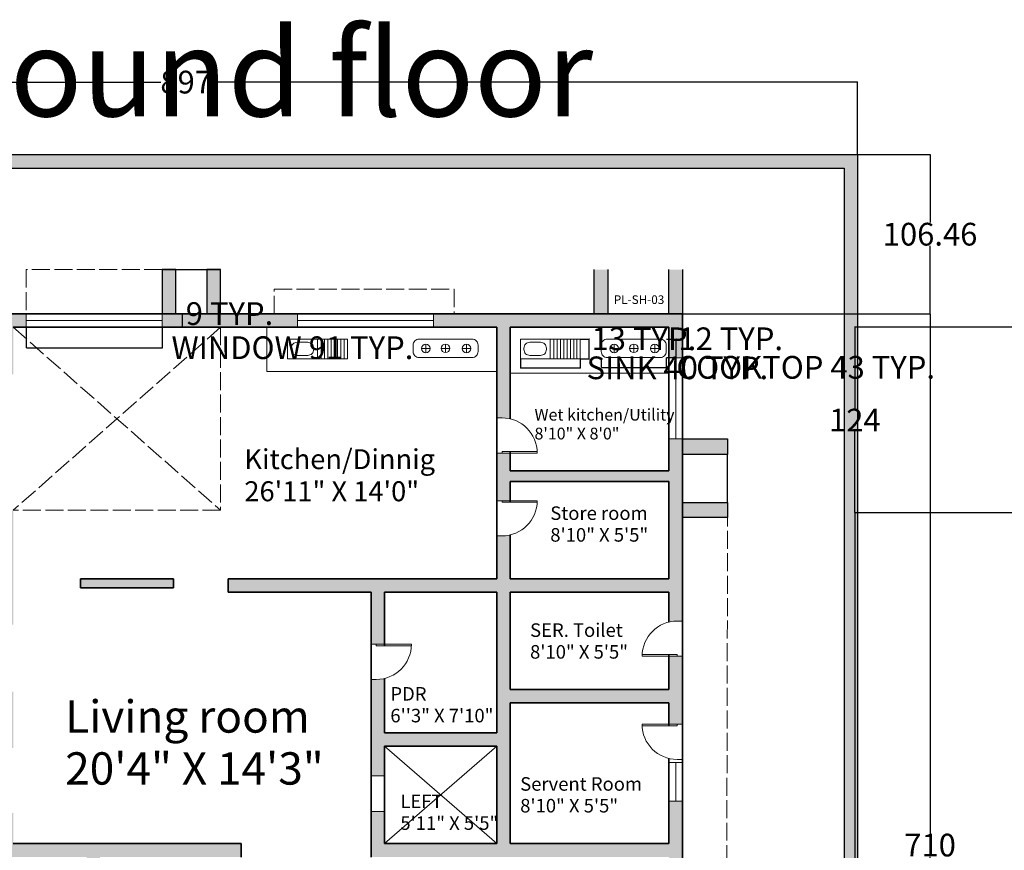
# Model space of a CAD drawing. Units: inches. Extents: x -828 to 1568, y -491 to 539.
# Tile 3 of 6: x -416 to 241, y -16 to 539. Entities that reach past the tile are written whole.
import ezdxf

# ---------------------------------------------------------------- set-up
doc = ezdxf.new("R2010")
doc.units = ezdxf.units.IN
doc.header["$MEASUREMENT"] = 0
doc.linetypes.add('ACAD_ISO02W100', pattern=[15, 12, -3])
for name, color, linetype, lineweight in [('A-ANNO-DIMS', 2, 'Continuous', 18), ('A-ANNO-TEXT', 7, 'Continuous', 18), ('A-ANNO-TITL', 7, 'Continuous', 35), ('A-AREA-IDEN', 7, 'Continuous', 18), ('A-DOOR', 3, 'Continuous', 18), ('A-EQPM', 9, 'Continuous', 18), ('A-FLOR-CASE', 9, 'Continuous', 18), ('A-FLOR-EVTR', 4, 'Continuous', 18), ('A-FLOR-FIXT', 9, 'Continuous', 18), ('A-FLOR-OVHD', 116, 'ACAD_ISO02W100', 13), ('A-FLOR-SHFT', 7, 'Continuous', 25), ('A-GLAZ', 4, 'Continuous', 18), ('A-WALL', 7, 'Continuous', 35), ('A-WALL-PATT', 8, 'Continuous', 13), ('L-SITE-PATT', 8, 'Continuous', 13), ('L-SITE-WALL', 7, 'Continuous', 30)]:
    doc.layers.add(name, color=color, linetype=linetype, lineweight=lineweight)
doc.styles.get("Standard").update_dxf_attribs({"font": 'arial.ttf'})
doc.dimstyles.get("Standard").update_dxf_attribs({"dimtxt": 15.18, "dimasz": 0.18, "dimexe": 0.18, "dimexo": 0.0625, "dimgap": 0.09, "dimtad": 0, "dimtih": 1, "dimtoh": 1, "dimdec": 0, "dimzin": 0, "dimdsep": 46, "dimlunit": 3, "dimtxsty": 'Standard', "dimcen": 0.09, "dimadec": 0, "dimazin": 0, "dimtfac": 1, "dimtdec": 0, "dimtofl": 0, "dimtmove": 0, "dimatfit": 3, "dimfxl": 1, "dimtolj": 1, "dimtzin": 0, "dimarcsym": 0})

# ---------------------------------------------------------------- blocks, each defined once
blk = doc.blocks.new('*U2')
for p, q in [((0, 0), (0, -6)), ((40, 0), (40, -6))]:
    blk.add_line(p, q)
blk.add_lwpolyline([(0, 0), (0, 40), (1.75, 40), (1.75, 0)], close=True)
blk.add_arc((0, 0), 40, 0, 90)
blk = doc.blocks.new('SINK-SINGLE-DRAINBOARD')
for p, q in [((0, 13.23), (40, 13.23)), ((0, 0), (0, 13.23)), ((20, 0), (20, 13.23)), ((22.4, 13.23), (22.4, 0)), ((24.6, 13.23), (24.6, 0)), ((26.8, 13.23), (26.8, 0)), ((29, 13.23), (29, 0)), ((31.2, 13.23), (31.2, 0)), ((33.4, 13.23), (33.4, 0)), ((35.6, 13.23), (35.6, 0)), ((37.8, 13.23), (37.8, 0)), ((40, 13.23), (40, 0)), ((20, 6.61), (20, 0)), ((40, 0), (0, 0))]:
    blk.add_line(p, q)
blk.add_lwpolyline([(6.36, 11.09), (13.4, 11.09, -0.414214), (17.4, 7.09), (17.4, 6.3, -0.414214), (13.4, 2.3), (6.36, 2.3, -0.414214), (2.36, 6.3), (2.36, 7.09, -0.414214)], format="xyb", close=True)
blk = doc.blocks.new('COOKTOP-3-BURNER')
for p, q in [((8.55, 6.06), (8.55, 8.95)), ((8.55, 8.95), (8.55, 3.17)), ((21.72, 6.18), (21.72, 9.07)), ((21.72, 9.07), (21.72, 3.29)), ((35.69, 6.06), (35.69, 8.95)), ((35.69, 8.95), (35.69, 3.17)), ((5.66, 6.06), (11.44, 6.06)), ((11.44, 6.06), (8.55, 6.06)), ((18.84, 6.18), (24.61, 6.18)), ((24.61, 6.18), (21.72, 6.18)), ((32.8, 6.06), (38.58, 6.06)), ((38.58, 6.06), (35.69, 6.06))]:
    blk.add_line(p, q)
blk.add_lwpolyline([(39.45, 0), (4, 0, -0.414214), (0, 4), (0, 8.37, -0.414214), (4, 12.37), (39.45, 12.37, -0.414214), (43.45, 8.37), (43.45, 4, -0.414214)], format="xyb", close=True)
for centre, radius in [((8.55, 6.06), 2.89), ((21.72, 6.18), 2.84), ((35.69, 6.06), 2.89)]:
    blk.add_circle(centre, radius)
blk = doc.blocks.new('WINDOW-90_84')
for p, q in [((0, 9), (0, 0)), ((90.84, 9), (0, 9)), ((90.84, 0), (90.84, 9)), ((0, 4.5), (90.84, 4.5)), ((0, 0), (90.84, 0))]:
    blk.add_line(p, q)
blk = doc.blocks.new('SERVICE-SHAFT-59')
for p, q in [((0, 49.77), (0, 58.98)), ((0, 58.98), (29.56, 58.98)), ((0, 58.98), (0, 0)), ((29.56, 49.77), (0, 49.77)), ((0, 0), (0, 9)), ((0, 9), (29.56, 9)), ((29.56, 0), (0, 0))]:
    blk.add_line(p, q)
blk = doc.blocks.new('*D15')
at = {"layer": 'A-ANNO-DIMS', "color": 0, "lineweight": -2, "transparency": 16777216}
for p, q in [((-81.78, 312.43), (-81.78, 306.32)), ((-41.78, 312.43), (-41.78, 306.32)), ((-81.6, 306.5), (-41.96, 306.5)), ((-41.78, 306.5), (-41.6, 306.5))]:
    blk.add_line(p, q, dxfattribs=at)
at = {"layer": 'A-ANNO-DIMS', "color": 0, "lineweight": 20, "transparency": 16777216}
for points in [[(-81.6, 306.53), (-81.6, 306.47), (-81.78, 306.5)], [(-41.96, 306.53), (-41.96, 306.47), (-41.78, 306.5)]]:
    blk.add_solid(points, dxfattribs=at)
at = {"layer": 'DEFPOINTS', "color": 0, "lineweight": 20, "transparency": 16777216}
for p in [(-81.78, 312.49), (-41.78, 312.49), (-41.78, 306.5)]:
    blk.add_point(p, dxfattribs=at)
at = {"layer": 'A-ANNO-DIMS', "color": 0, "transparency": 16777216, "insert": (23.09, 306.5), "char_height": 15.18, "attachment_point": 5}
blk.add_mtext('\\A1;SINK 40 TYP.', dxfattribs=at)
blk = doc.blocks.new('*D16')
at = {"layer": 'A-ANNO-DIMS', "color": 0, "lineweight": -2, "transparency": 16777216}
for p, q in [((-41.72, 325.73), (-35.6, 325.73)), ((-35.78, 325.73), (-35.78, 325.91)), ((-35.78, 325.91), (-35.6, 325.91)), ((-35.78, 312.67), (-35.78, 325.55)), ((-41.72, 312.49), (-35.6, 312.49))]:
    blk.add_line(p, q, dxfattribs=at)
at = {"layer": 'A-ANNO-DIMS', "color": 0, "lineweight": 20, "transparency": 16777216}
for points in [[(-35.81, 325.55), (-35.75, 325.55), (-35.78, 325.73)], [(-35.81, 312.67), (-35.75, 312.67), (-35.78, 312.49)]]:
    blk.add_solid(points, dxfattribs=at)
at = {"layer": 'DEFPOINTS', "color": 0, "lineweight": 20, "transparency": 16777216}
for p in [(-41.78, 325.73), (-35.78, 325.73), (-41.78, 312.49)]:
    blk.add_point(p, dxfattribs=at)
at = {"layer": 'A-ANNO-DIMS', "color": 0, "transparency": 16777216, "insert": (0.72, 325.91), "char_height": 15.18, "attachment_point": 5}
blk.add_mtext('\\A1;13 TYP.', dxfattribs=at)
blk = doc.blocks.new('*D17')
at = {"layer": 'A-ANNO-DIMS', "color": 0, "lineweight": -2, "transparency": 16777216}
for p, q in [((-27.75, 313.3), (-27.75, 306.66)), ((15.7, 313.3), (15.7, 306.66)), ((-27.57, 306.84), (15.52, 306.84)), ((15.7, 306.84), (15.88, 306.84))]:
    blk.add_line(p, q, dxfattribs=at)
at = {"layer": 'A-ANNO-DIMS', "color": 0, "lineweight": 20, "transparency": 16777216}
for points in [[(-27.57, 306.87), (-27.57, 306.81), (-27.75, 306.84)], [(15.52, 306.87), (15.52, 306.81), (15.7, 306.84)]]:
    blk.add_solid(points, dxfattribs=at)
at = {"layer": 'DEFPOINTS', "color": 0, "lineweight": 20, "transparency": 16777216}
for p in [(-27.75, 313.36), (15.7, 313.36), (15.7, 306.84)]:
    blk.add_point(p, dxfattribs=at)
at = {"layer": 'A-ANNO-DIMS', "color": 0, "transparency": 16777216, "insert": (108.8, 306.84), "char_height": 15.18, "attachment_point": 5}
blk.add_mtext('\\A1;COOKTOP 43 TYP.', dxfattribs=at)
blk = doc.blocks.new('*D18')
at = {"layer": 'A-ANNO-DIMS', "color": 0, "lineweight": -2, "transparency": 16777216}
for p, q in [((15.77, 325.73), (22.4, 325.73)), ((22.22, 325.73), (22.22, 325.91)), ((22.22, 325.91), (22.4, 325.91)), ((22.22, 313.54), (22.22, 325.55)), ((15.77, 313.36), (22.4, 313.36))]:
    blk.add_line(p, q, dxfattribs=at)
at = {"layer": 'A-ANNO-DIMS', "color": 0, "lineweight": 20, "transparency": 16777216}
for points in [[(22.19, 325.55), (22.25, 325.55), (22.22, 325.73)], [(22.19, 313.54), (22.25, 313.54), (22.22, 313.36)]]:
    blk.add_solid(points, dxfattribs=at)
at = {"layer": 'DEFPOINTS', "color": 0, "lineweight": 20, "transparency": 16777216}
for p in [(15.7, 325.73), (22.22, 325.73), (15.7, 313.36)]:
    blk.add_point(p, dxfattribs=at)
at = {"layer": 'A-ANNO-DIMS', "color": 0, "transparency": 16777216, "insert": (58.72, 325.91), "char_height": 15.18, "attachment_point": 5}
blk.add_mtext('\\A1;12 TYP.', dxfattribs=at)
blk = doc.blocks.new('*D19')
at = {"layer": 'A-ANNO-DIMS', "color": 0, "lineweight": -2, "transparency": 16777216}
for p, q in [((-411.88, 333.52), (-411.88, 319.78)), ((-321.03, 333.52), (-321.03, 319.78)), ((-411.7, 319.96), (-321.21, 319.96)), ((-321.03, 319.96), (-320.85, 319.96))]:
    blk.add_line(p, q, dxfattribs=at)
at = {"layer": 'A-ANNO-DIMS', "color": 0, "lineweight": 20, "transparency": 16777216}
for points in [[(-411.7, 319.99), (-411.7, 319.93), (-411.88, 319.96)], [(-321.21, 319.99), (-321.21, 319.93), (-321.03, 319.96)]]:
    blk.add_solid(points, dxfattribs=at)
at = {"layer": 'DEFPOINTS', "color": 0, "lineweight": 20, "transparency": 16777216}
for p in [(-411.88, 333.58), (-321.03, 333.58), (-321.03, 319.96)]:
    blk.add_point(p, dxfattribs=at)
at = {"layer": 'A-ANNO-DIMS', "color": 0, "transparency": 16777216, "insert": (-234.04, 319.96), "char_height": 15.18, "attachment_point": 5}
blk.add_mtext('\\A1;WINDOW 91 TYP.', dxfattribs=at)
blk = doc.blocks.new('*D20')
at = {"layer": 'A-ANNO-DIMS', "color": 0, "lineweight": -2, "transparency": 16777216}
for p, q in [((-320.97, 342.58), (-307.23, 342.58)), ((-307.41, 342.58), (-307.41, 342.76)), ((-307.41, 342.76), (-307.23, 342.76)), ((-307.41, 333.76), (-307.41, 342.4)), ((-320.97, 333.58), (-307.23, 333.58))]:
    blk.add_line(p, q, dxfattribs=at)
at = {"layer": 'A-ANNO-DIMS', "color": 0, "lineweight": 20, "transparency": 16777216}
for points in [[(-307.44, 342.4), (-307.38, 342.4), (-307.41, 342.58)], [(-307.44, 333.76), (-307.38, 333.76), (-307.41, 333.58)]]:
    blk.add_solid(points, dxfattribs=at)
at = {"layer": 'DEFPOINTS', "color": 0, "lineweight": 20, "transparency": 16777216}
for p in [(-321.03, 342.58), (-307.41, 342.58), (-321.03, 333.58)]:
    blk.add_point(p, dxfattribs=at)
at = {"layer": 'A-ANNO-DIMS', "color": 0, "transparency": 16777216, "insert": (-276.09, 342.76), "char_height": 15.18, "attachment_point": 5}
blk.add_mtext('\\A1;9 TYP.', dxfattribs=at)
blk = doc.blocks.new('*D31')
at = {"layer": 'A-ANNO-DIMS', "color": 0, "lineweight": -2, "transparency": 16777216}
for p, q in [((-753.52, 449.11), (-753.52, 497.62)), ((-753.34, 497.44), (-321.89, 497.44)), ((143.29, 497.44), (-288.15, 497.44)), ((143.47, 449.11), (143.47, 497.62))]:
    blk.add_line(p, q, dxfattribs=at)
at = {"layer": 'A-ANNO-DIMS', "color": 0, "lineweight": 20, "transparency": 16777216}
for points in [[(-753.34, 497.47), (-753.34, 497.41), (-753.52, 497.44)], [(143.29, 497.47), (143.29, 497.41), (143.47, 497.44)]]:
    blk.add_solid(points, dxfattribs=at)
at = {"layer": 'DEFPOINTS', "color": 0, "lineweight": 20, "transparency": 16777216}
for p in [(143.47, 497.44), (-753.52, 449.04), (143.47, 449.04)]:
    blk.add_point(p, dxfattribs=at)
at = {"layer": 'A-ANNO-DIMS', "color": 0, "transparency": 16777216, "insert": (-305.02, 497.44), "char_height": 15.18, "attachment_point": 5}
blk.add_mtext('\\A1;897', dxfattribs=at)
blk = doc.blocks.new('*D34')
at = {"layer": 'A-ANNO-DIMS', "color": 0, "lineweight": -2, "transparency": 16777216}
for p, q in [((26.52, 342.58), (192.05, 342.58)), ((191.87, 342.4), (191.87, -4.57)), ((191.87, -367.24), (191.87, -20.26)), ((26.52, -367.42), (192.05, -367.42))]:
    blk.add_line(p, q, dxfattribs=at)
at = {"layer": 'A-ANNO-DIMS', "color": 0, "lineweight": 20, "transparency": 16777216}
for points in [[(191.84, 342.4), (191.9, 342.4), (191.87, 342.58)], [(191.84, -367.24), (191.9, -367.24), (191.87, -367.42)]]:
    blk.add_solid(points, dxfattribs=at)
at = {"layer": 'DEFPOINTS', "color": 0, "lineweight": 20, "transparency": 16777216}
for p in [(26.46, 342.58), (191.87, 342.58), (26.46, -367.42)]:
    blk.add_point(p, dxfattribs=at)
at = {"layer": 'A-ANNO-DIMS', "color": 0, "transparency": 16777216, "insert": (191.87, -12.42), "char_height": 15.18, "attachment_point": 5}
blk.add_mtext('\\A1;710', dxfattribs=at)
blk = doc.blocks.new('*D36')
at = {"layer": 'A-ANNO-DIMS', "color": 0, "lineweight": -2, "transparency": 16777216}
for p, q in [((143.54, 449.04), (192.05, 449.04)), ((191.87, 448.86), (191.87, 403.65)), ((191.87, 342.76), (191.87, 387.97)), ((26.52, 342.58), (192.05, 342.58))]:
    blk.add_line(p, q, dxfattribs=at)
at = {"layer": 'A-ANNO-DIMS', "color": 0, "lineweight": 20, "transparency": 16777216}
for points in [[(191.84, 448.86), (191.9, 448.86), (191.87, 449.04)], [(191.84, 342.76), (191.9, 342.76), (191.87, 342.58)]]:
    blk.add_solid(points, dxfattribs=at)
at = {"layer": 'DEFPOINTS', "color": 0, "lineweight": 20, "transparency": 16777216}
for p in [(143.47, 449.04), (26.46, 342.58), (191.87, 342.58)]:
    blk.add_point(p, dxfattribs=at)
at = {"layer": 'A-ANNO-DIMS', "color": 0, "transparency": 16777216, "insert": (191.87, 395.81), "char_height": 15.18, "attachment_point": 5}
blk.add_mtext('\\A1;106.46', dxfattribs=at)
blk = doc.blocks.new('*D42')
at = {"layer": 'A-ANNO-DIMS', "color": 0, "lineweight": -2, "transparency": 16777216}
for p, q in [((347.86, 209.58), (141.48, 209.58)), ((141.66, 209.4), (141.66, -76.07)), ((141.66, -377.24), (141.66, -91.76)), ((279.86, -377.42), (141.48, -377.42))]:
    blk.add_line(p, q, dxfattribs=at)
at = {"layer": 'A-ANNO-DIMS', "color": 0, "lineweight": 20, "transparency": 16777216}
for points in [[(141.63, 209.4), (141.69, 209.4), (141.66, 209.58)], [(141.63, -377.24), (141.69, -377.24), (141.66, -377.42)]]:
    blk.add_solid(points, dxfattribs=at)
at = {"layer": 'DEFPOINTS', "color": 0, "lineweight": 20, "transparency": 16777216}
for p in [(141.66, 209.58), (347.92, 209.58), (279.92, -377.42)]:
    blk.add_point(p, dxfattribs=at)
at = {"layer": 'A-ANNO-DIMS', "color": 0, "transparency": 16777216, "insert": (141.66, -83.92), "char_height": 15.18, "attachment_point": 5}
blk.add_mtext('\\A1;587', dxfattribs=at)
blk = doc.blocks.new('*D44')
at = {"layer": 'A-ANNO-DIMS', "color": 0, "lineweight": -2, "transparency": 16777216}
for p, q in [((347.86, 333.58), (141.48, 333.58)), ((141.66, 333.4), (141.66, 279.3)), ((141.66, 209.76), (141.66, 263.87)), ((347.86, 209.58), (141.48, 209.58))]:
    blk.add_line(p, q, dxfattribs=at)
at = {"layer": 'A-ANNO-DIMS', "color": 0, "lineweight": 20, "transparency": 16777216}
for points in [[(141.63, 333.4), (141.69, 333.4), (141.66, 333.58)], [(141.63, 209.76), (141.69, 209.76), (141.66, 209.58)]]:
    blk.add_solid(points, dxfattribs=at)
at = {"layer": 'DEFPOINTS', "color": 0, "lineweight": 20, "transparency": 16777216}
for p in [(141.66, 333.58), (347.92, 333.58), (347.92, 209.58)]:
    blk.add_point(p, dxfattribs=at)
at = {"layer": 'A-ANNO-DIMS', "color": 0, "transparency": 16777216, "insert": (141.66, 271.58), "char_height": 15.18, "attachment_point": 5}
blk.add_mtext('\\A1;124', dxfattribs=at)

msp = doc.modelspace()

# ---------------------------------------------------------------- hatches: boundary and pattern name
at = {"layer": 'A-WALL-PATT'}
h = msp.add_hatch(color=256, dxfattribs=at)
h.dxf.hatch_style = 1
h.paths.add_polyline_path([(-473.7903, -197.4155), (-523.4337, -197.4155), (-523.4337, -206.4155), (-473.7903, -206.4155)])
h.paths.add_polyline_path([(-572.3651, -197.4155), (-595.5391, -197.4155), (-595.5391, -20.4155), (-520.2134, -20.4155), (-520.2134, -11.4155), (-604.5391, -11.4155), (-604.5391, -206.4155), (-572.3651, -206.4155)])
h.paths.add_polyline_path([(-604.5391, -170.4394), (-634.1027, -170.4394), (-634.1027, -179.4394), (-604.5391, -179.4394)])
h.paths.add_polyline_path([(-604.5391, -120.4631), (-634.1027, -120.4631), (-634.1027, -129.6673), (-604.5391, -129.6673)])
h.paths.add_polyline_path([(-268.3198, -11.4155), (-420.5391, -11.4155), (-420.5391, 9.0334), (-429.5391, 9.0334), (-429.5391, -11.4155), (-471.2821, -11.4155), (-471.2821, -20.4155), (-371.5391, -20.4155), (-371.5391, -197.4155), (-400.5108, -197.4155), (-400.5108, -206.4155), (-371.5391, -206.4155), (-371.5391, -282.4155), (-367.0391, -282.4155), (-362.5391, -282.4155), (-362.5391, -122.4155), (-313.1564, -122.4155), (-313.1564, -113.4155), (-362.5391, -113.4155), (-362.5391, -20.4155), (-268.3198, -20.4155)])
h.paths.add_polyline_path([(-313.539, 165.5845), (-375.5295, 165.5845), (-375.5295, 159.5845), (-313.539, 159.5845)])
h.paths.add_polyline_path([(-420.5391, 90.211), (-429.5391, 90.211), (-429.5391, 52.4437), (-420.5391, 52.4437)])
h.paths.add_polyline_path([(-420.5391, 211.3197), (-429.5391, 211.3197), (-429.5391, 134.8496), (-425.0391, 134.8496), (-420.5391, 134.8496), (-420.5391, 165.5845)])
h.paths.add_polyline_path([(-429.5391, 188.7113), (-438.5391, 188.7113), (-438.5391, 145.3797), (-429.5391, 145.3797)])
h.paths.add_polyline_path([(-517.0391, 342.5845), (-604.5391, 342.5845), (-604.5391, 333.5845), (-517.0391, 333.5845)])
h.paths.add_polyline_path([(-411.8784, 342.5845), (-429.5391, 342.5845), (-429.5391, 302.1645), (-420.5391, 302.1645), (-420.5391, 333.5845), (-411.8784, 333.5845)])
h.paths.add_polyline_path([(-311.8294, 372.1481), (-321.0336, 372.1481), (-321.0336, 342.5845), (-311.8294, 342.5845)])
h.paths.add_polyline_path([(-282.0163, 372.1481), (-291.2206, 372.1481), (-291.2206, 342.5845), (-282.0163, 342.5845)])
h.paths.add_polyline_path([(-230.7265, 342.5845), (-321.0336, 342.5845), (-321.0336, 333.5845), (-230.7265, 333.5845)])
h.paths.add_polyline_path([(-23.3113, 372.1481), (-32.5155, 372.1481), (-32.5155, 342.5845), (-23.3113, 342.5845)])
h.paths.add_polyline_path([(26.4609, 372.1481), (17.4609, 372.1481), (17.4609, 342.5845), (26.4609, 342.5845)])
h.paths.add_polyline_path([(56.6461, 259.1031), (26.4609, 259.1031), (26.4609, 248.5663), (56.6461, 248.5663)])
h.paths.add_polyline_path([(56.6461, 216.517), (26.4609, 216.517), (26.4609, 206.4193), (56.6461, 206.4193)])
h.paths.add_polyline_path([(56.0244, -54.4391), (26.4609, -54.4391), (26.4609, -63.6433), (56.0244, -63.6433)])
h.paths.add_polyline_path([(56.0244, -163.1876), (26.4609, -163.1876), (26.4609, -172.3918), (56.0244, -172.3918)])
h.paths.add_polyline_path([(56.0244, -113.4155), (56.0244, -104.4155), (26.4609, -104.4155), (26.4609, -122.4155), (56.0244, -122.4155)])
h.paths.add_polyline_path([(-23.844, -367.4155), (-134.8372, -367.4155), (-134.8372, -376.4155), (-23.844, -376.4155)])
h.paths.add_polyline_path([(26.4609, -54.4391), (21.9609, -54.4391), (17.4609, -54.4391), (17.4609, -113.4155), (-252.861, -113.4155), (-252.861, -122.4155), (-69.5391, -122.4155), (-69.5391, -282.9566), (-65.5391, -282.9566), (-65.5391, -250.4155), (-53.4738, -250.4155), (-53.4738, -246.4155), (-65.5391, -246.4155), (-65.5391, -122.4155), (17.4609, -122.4155), (17.4609, -172.3918), (26.4609, -172.3918), (26.4609, -163.1876)])
h.paths.add_polyline_path([(-172.5391, 156.5845), (-97.5391, 156.5845), (-97.5391, 62.5845), (-172.5391, 62.5845), (-172.5391, 98.9611, -0.05899862), (-178.0193, 98.3122), (-181.5391, 98.3122), (-181.5391, 33.9683), (-172.5391, 33.9683), (-172.5391, 53.5845), (-97.5391, 53.5845), (-97.5391, -11.4155), (-172.5391, -11.4155), (-172.5391, 9.9791), (-181.5391, 9.9791), (-181.5391, -11.4155), (-181.5391, -20.4155), (17.4609, -20.4155), (17.4609, -29.0707), (26.4609, -29.0707), (26.4609, 17.0407), (17.4609, 17.0407), (17.4609, -11.4155), (-88.5391, -11.4155), (-88.5391, 82.5845), (17.4609, 82.5845), (17.4609, 68.3133), (22.9411, 68.3133), (26.4609, 68.3133), (26.4609, 113.8123), (23.0131, 113.8123), (17.4609, 113.8123), (17.4609, 91.5845), (-88.5391, 91.5845), (-88.5391, 156.5845), (17.4609, 156.5845), (17.4609, 136.6113, -0.05979118), (23.0131, 137.2776), (26.4609, 137.2776), (26.4609, 259.1031), (21.9609, 259.1031), (17.4609, 259.1031), (17.4609, 237.5845), (-88.5391, 237.5845), (-88.5391, 249.5845), (-94.0193, 249.5845), (-97.5391, 249.5845), (-97.5391, 217.6678), (-94.0193, 217.6678), (-88.5391, 217.6678), (-88.5391, 230.5845), (17.4609, 230.5845), (17.4609, 165.5845), (-88.5391, 165.5845), (-88.5391, 194.8514, -0.05899862), (-94.0193, 194.2024), (-97.5391, 194.2024), (-97.5391, 165.5845), (-276.9691, 165.5845), (-276.9691, 156.5845), (-181.5391, 156.5845), (-181.5391, 121.7776), (-178.0193, 121.7776), (-172.5391, 121.7776)])
h.paths.add_polyline_path([(-88.5391, 333.5845), (17.4609, 333.5845), (17.4609, 313.1897), (26.4609, 313.1897), (26.4609, 342.5845), (-139.8817, 342.5845), (-139.8817, 333.5845), (-97.5391, 333.5845), (-97.5391, 273.0499), (-94.0193, 273.0499, -0.05899862), (-88.5391, 272.401)])
h.paths.add_polyline_path([(26.4609, -232.3042), (17.4609, -232.3042), (17.4609, -246.4155), (-35.2489, -246.4155), (-35.2489, -250.4155), (17.4609, -250.4155), (17.4609, -358.4155), (-65.5391, -358.4155), (-65.5391, -311.3725), (-69.5391, -311.3725), (-69.5391, -358.4155), (-261.1271, -358.4155), (-261.1271, -367.4155), (26.4609, -367.4155)])
at = {"layer": 'L-SITE-PATT'}
h = msp.add_hatch(color=256, dxfattribs=at)
h.dxf.hatch_style = 1
h.paths.add_polyline_path([(-695.1383, -418.734), (-695.1383, -409.734), (-744.5156, -409.734), (-744.5156, 440.0429), (134.4735, 440.0429), (134.4735, -409.734), (-428.0987, -409.734), (-428.0987, -418.734), (143.4735, -418.734), (143.4735, 449.0429), (-753.5156, 449.0429), (-753.5156, -418.734)])

# ---------------------------------------------------------------- linework, layer by layer
at = {"layer": 'A-FLOR-CASE'}
msp.add_line((-88.5391, 302.9928), (17.4609, 302.9928), dxfattribs=at)
msp.add_lwpolyline([(-97.5391, 333.5845), (-251.1423, 333.5845), (-251.1423, 304.1078), (-97.5391, 304.1078)], close=True, dxfattribs=at)
at = {"layer": 'A-FLOR-EVTR'}
for p, q in [((-172.5391, -11.4155), (-97.5391, 53.5845)), ((-97.5391, -11.4155), (-172.5391, 53.5845)), ((-97.5391, 53.5845), (-97.5391, -11.4155)), ((-172.5391, 33.9683), (-181.5391, 33.9683)), ((-181.5391, 33.9683), (-181.5391, 9.9791)), ((-181.5391, 9.9791), (-181.5391, 9.9791)), ((-181.5391, 9.9791), (-172.5391, 9.9791))]:
    msp.add_line(p, q, dxfattribs=at)
at = {"layer": 'A-FLOR-OVHD'}
for p, q in [((-321.0336, 372.1481), (-411.8784, 372.1481)), ((-411.8784, 372.1481), (-411.8784, 342.5845)), ((-246.3192, 342.5845), (-246.3192, 359.1397)), ((-246.3192, 359.1397), (-125.9568, 359.1397)), ((-125.9568, 359.1397), (-125.9568, 342.5845)), ((-420.5391, 333.5845), (-282.0163, 333.5845)), ((-282.0163, 333.5845), (-420.5391, 211.3197)), ((-420.5391, 333.5845), (-282.0163, 211.3197)), ((-282.0163, 333.5845), (-282.0163, 211.3197)), ((-282.0163, 211.3197), (-420.5391, 211.3197)), ((56.0244, -54.4391), (56.6461, 206.4193))]:
    msp.add_line(p, q, dxfattribs=at)
at = {"layer": 'A-FLOR-SHFT'}
for p, q in [((-311.8294, 372.1481), (-321.0336, 372.1481)), ((-321.0336, 372.1481), (-321.0336, 342.5845)), ((-321.0336, 372.1481), (-282.0163, 372.1481)), ((-311.8294, 342.5845), (-311.8294, 372.1481)), ((-282.0163, 372.1481), (-291.2206, 372.1481)), ((-291.2206, 372.1481), (-291.2206, 342.5845)), ((-282.0163, 342.5845), (-282.0163, 372.1481)), ((-32.5155, 342.5845), (26.4609, 342.5845)), ((17.4609, 342.5845), (-23.3113, 342.5845)), ((26.4609, 342.5845), (17.4609, 342.5845)), ((26.4609, 259.1031), (56.6461, 259.1031)), ((56.6461, 259.1031), (56.6461, 248.5663)), ((56.6461, 248.5663), (26.4609, 248.5663)), ((56.6461, 216.517), (56.6461, 248.5663)), ((26.4609, 216.517), (56.6461, 216.517)), ((26.4609, 216.517), (56.6461, 216.517)), ((56.6461, 216.517), (56.6461, 206.4193)), ((56.6461, 206.4193), (26.4609, 206.4193)), ((26.4609, 165.5845), (26.4609, 191.7262)), ((26.4609, 181.1894), (26.4609, 149.1401)), ((26.4609, 139.0424), (26.4609, 149.1401))]:
    msp.add_line(p, q, dxfattribs=at)
at = {"layer": 'A-GLAZ'}
for p, q in [((17.4609, 259.1031), (17.4609, 313.1897)), ((17.4609, 313.1897), (26.4609, 313.1897)), ((21.9609, 259.1031), (21.9609, 313.1897)), ((26.4609, 313.1897), (26.4609, 259.1031)), ((26.4609, 259.1031), (17.4609, 259.1031)), ((26.4609, 259.1031), (21.9609, 259.1031)), ((26.4609, 42.74), (17.4609, 42.74)), ((17.4609, 42.74), (17.4609, 17.0407)), ((26.4609, 42.74), (21.9609, 42.74)), ((21.9609, 42.74), (21.9609, 17.0407)), ((26.4609, 17.0407), (26.4609, 42.74)), ((17.4609, 17.0407), (26.4609, 17.0407))]:
    msp.add_line(p, q, dxfattribs=at)
at = {"layer": 'A-WALL'}
for p, q in [((26.4609, 342.5845), (-429.5391, 342.5845)), ((26.4609, 342.5845), (26.4609, -367.4155)), ((-97.5391, 333.5845), (-420.5391, 333.5845)), ((-97.5391, 333.5845), (-97.5391, 165.5845)), ((-88.5391, 333.5845), (-88.5391, 272.401)), ((17.4609, 333.5845), (-88.5391, 333.5845)), ((-88.5391, 333.5845), (17.4609, 333.5845)), ((17.4609, 333.5845), (17.4609, 237.5845)), ((-88.5391, 250.6111), (-88.5391, 237.5845)), ((-88.5391, 237.5845), (17.4609, 237.5845)), ((-88.5391, 230.5845), (17.4609, 230.5845)), ((-88.5391, 230.5845), (-88.5391, 216.6412)), ((17.4609, 230.5845), (17.4609, 165.5845)), ((-88.5391, 194.8514), (-88.5391, 165.5845)), ((-313.539, 165.5845), (-375.5295, 165.5845)), ((-375.5295, 165.5845), (-375.5295, 159.5845)), ((-313.539, 165.5845), (-313.539, 159.5845)), ((-97.5391, 165.5845), (-276.9691, 165.5845)), ((-276.9691, 165.5845), (-276.9691, 156.5845)), ((17.4609, 165.5845), (-88.5391, 165.5845)), ((-88.5391, 165.5845), (17.4609, 165.5845)), ((-375.5295, 159.5845), (-313.539, 159.5845)), ((-181.5391, 156.5845), (-276.9691, 156.5845)), ((-181.5391, 156.5845), (-181.5391, -11.4155)), ((-172.5391, 156.5845), (-172.5391, 120.751)), ((-172.5391, 156.5845), (-97.5391, 156.5845)), ((-97.5391, 156.5845), (-172.5391, 156.5845)), ((-97.5391, 156.5845), (-97.5391, 62.5845)), ((-97.5391, 156.5845), (-97.5391, 62.5845)), ((17.4609, 156.5845), (-88.5391, 156.5845)), ((-88.5391, 156.5845), (17.4609, 156.5845)), ((-88.5391, 156.5845), (-88.5391, 91.5845)), ((17.4609, 156.5845), (17.4609, 136.6113)), ((17.4609, 114.8389), (17.4609, 91.5845)), ((-172.5391, 98.9611), (-172.5391, 62.5845)), ((-88.5391, 91.5845), (17.4609, 91.5845)), ((-88.5391, 82.5845), (17.4609, 82.5845)), ((-88.5391, 82.5845), (-88.5391, -11.4155)), ((17.4609, 82.5845), (17.4609, 67.2867)), ((-172.5391, 62.5845), (-97.5391, 62.5845)), ((-172.5391, 53.5845), (-97.5391, 53.5845)), ((-172.5391, 53.5845), (-172.5391, -11.4155)), ((-97.5391, 53.5845), (-97.5391, -11.4155)), ((-97.5391, 53.5845), (-97.5391, -11.4155)), ((17.4609, 45.4969), (17.4609, -11.4155)), ((-420.5391, -11.4155), (-268.3198, -11.4155)), ((-268.3198, -11.4155), (-268.3198, -11.4155)), ((-268.3198, -11.4155), (-268.3198, -20.4155)), ((-181.5391, -11.4155), (-181.5391, -20.4155)), ((-172.5391, -11.4155), (-97.5391, -11.4155)), ((-88.5391, -11.4155), (17.4609, -11.4155))]:
    msp.add_line(p, q, dxfattribs=at)
at = {"layer": 'L-SITE-WALL'}
for points in [[(-695.1383, -418.734), (-753.5156, -418.734), (-753.5156, 449.0429), (143.4735, 449.0429), (143.4735, -418.734), (-548.5793, -418.734)], [(-695.1383, -409.734), (-744.5156, -409.734), (-744.5156, 440.0429), (134.4735, 440.0429), (134.4735, -409.734), (-548.5793, -409.734)]]:
    msp.add_lwpolyline(points, dxfattribs=at)

# ---------------------------------------------------------------- block references
at = {"layer": 'A-DOOR', "yscale": 0.5866336421401575, "zscale": 0.5866336421401575}
for p, xscale, rotation in [((-94.0193, 249.5845), -0.5866336421401575, 270), ((-94.0193, 217.6678), 0.5866336421401575, 270), ((23.0131, 113.8123), 0.5866336421401575, 89.99999999999999), ((-178.0193, 121.7776), 0.5866336421401575, 270), ((22.9411, 68.3133), -0.5866336421401575, 90)]:
    msp.add_blockref('*U2', p, dxfattribs=dict(at, xscale=xscale, rotation=rotation))
at = {"layer": 'A-EQPM'}
for p in [(-153.498, 313.358), (-27.7458, 313.358)]:
    msp.add_blockref('COOKTOP-3-BURNER', p, dxfattribs=at)
at = {"layer": 'A-FLOR-FIXT'}
for p in [(-237.232, 312.495), (-81.7787, 312.495)]:
    msp.add_blockref('SINK-SINGLE-DRAINBOARD', p, dxfattribs=at)
at = {"layer": 'A-FLOR-SHFT', "rotation": 90}
msp.add_blockref('SERVICE-SHAFT-59', (26.4604, 342.5842), dxfattribs=at)
at = {"layer": 'A-GLAZ'}
msp.add_blockref('WINDOW-90_84', (-411.878, 333.585), dxfattribs=at)
at = {"layer": 'A-GLAZ', "rotation": 180}
msp.add_blockref('WINDOW-90_84', (-139.8821, 342.5841), dxfattribs=at)

# ---------------------------------------------------------------- texts
at = {"layer": 'A-ANNO-TEXT'}
msp.add_text('PL-SH-03', height=5.74254, dxfattribs=at).set_placement((-19.374, 349.1834))
at = {"layer": 'A-ANNO-TITL'}
msp.add_text('Ground floor', height=58.547339, dxfattribs=at).set_placement((-508.7568, 474.5437))
at = {"layer": 'A-AREA-IDEN'}
for s, height, p in [('Wet kitchen/Utility', 7.84507, (-72.3644, 271.2623)), ('8\'10" X 8\'0"', 7.84507, (-72.3644, 258.6598)), ('Kitchen/Dinnig', 13.349325, (-266.1291, 238.7936)), ('26\'11" X 14\'0"', 13.349325, (-266.1291, 217.349)), ('Store room', 9.04554, (-61.801, 204.8751)), ('8\'10" X 5\'5"', 9.045542, (-61.801, 190.3442)), ('SER. Toilet', 9.045542, (-75.3019, 126.7095)), ('8\'10" X 5\'5"', 9.045542, (-75.3019, 112.1786)), ('PDR', 9.04554, (-168.6126, 84.1267)), ('Living room', 21.617789, (-385.8084, 62.7096)), ('6\'\'3" X 7\'10"', 9.045542, (-168.6126, 69.5959)), ('20\'4" X 14\'3"', 21.617789, (-385.8084, 27.9826)), ('Servent Room', 9.045542, (-81.9071, 23.9212)), ('LEFT', 9.04554, (-161.9504, 12.2923)), ('8\'10" X 5\'5"', 9.045542, (-81.9071, 9.3903)), ('5\'11" X 5\'5"', 9.045542, (-161.9504, -2.2386))]:
    msp.add_text(s, height=height, dxfattribs=at).set_placement(p)

# ---------------------------------------------------------------- dimensions: what is measured, and where the dimension line sits
at = {"layer": 'A-ANNO-DIMS'}
dim = msp.add_linear_dim(base=(143.4735, 497.4429), p1=(-753.5156, 449.0429), p2=(143.4735, 449.0429), dimstyle='Standard', override={"dimdec": 0, "dimlfac": 1, "dimrnd": 0, "dimzin": 0, "dimdsep": 46, "dimlunit": 2}, dxfattribs=at)
dim.commit()
dim.dimension.update_dxf_attribs({"geometry": '*D31', "text_midpoint": (-305.0211, 497.4429)})
for base, p1, p2, override, picture, middle in [((191.8735, 342.5845), (143.4735, 449.0429), (26.4609, 342.5845), {"dimdec": 2, "dimlfac": 1, "dimrnd": 0, "dimzin": 0, "dimdsep": 46, "dimlunit": 2}, '*D36', (191.8735, 395.8137)), ((191.8735, 342.5845), (26.4609, -367.4155), (26.4609, 342.5845), {"dimdec": 0, "dimlfac": 1, "dimrnd": 0, "dimzin": 0, "dimdsep": 46, "dimlunit": 2}, '*D34', (191.8735, -12.4155)), ((141.6607, 333.5845), (347.9226, 209.5845), (347.9226, 333.5845), {"dimdec": 0, "dimlfac": 1, "dimrnd": 0, "dimzin": 0, "dimdsep": 46, "dimlunit": 2}, '*D44', (141.6607, 271.5845)), ((141.6607, 209.5845), (279.9226, -377.4155), (347.9226, 209.5845), {"dimdec": 0, "dimlfac": 1, "dimrnd": 0, "dimzin": 0, "dimdsep": 46, "dimlunit": 2}, '*D42', (141.6607, -83.9155))]:
    dim = msp.add_linear_dim(base=base, p1=p1, p2=p2, angle=90, dimstyle='Standard', override=override, dxfattribs=at)
    dim.commit()
    dim.dimension.update_dxf_attribs({"geometry": picture, "text_midpoint": middle})
for base, p1, p2, picture, middle in [((-307.4069, 342.5845), (-321.0336, 333.5845), (-321.0336, 342.5845), '*D20', (-276.0883, 342.7645)), ((-35.7825, 325.7251), (-41.782, 312.4948), (-41.782, 325.7251), '*D16', (0.7186, 325.9051)), ((22.2205, 325.7251), (15.7031, 313.3576), (15.7031, 325.7251), '*D18', (58.7216, 325.9051))]:
    dim = msp.add_linear_dim(base=base, p1=p1, p2=p2, angle=90, text='<> TYP.', dimstyle='Standard', override={"dimdec": 0, "dimlfac": 1, "dimrnd": 0, "dimzin": 0, "dimdsep": 46, "dimlunit": 2}, dxfattribs=at)
    dim.commit()
    dim.dimension.update_dxf_attribs({"geometry": picture, "text_midpoint": middle})
for base, p1, p2, text, picture, middle in [((-321.0336, 319.9578), (-411.8784, 333.5845), (-321.0336, 333.5845), 'WINDOW <> TYP.', '*D19', (-234.0378, 319.9578)), ((15.7031, 306.8402), (-27.7461, 313.3576), (15.7031, 313.3576), 'COOKTOP <> TYP.', '*D17', (108.7979, 306.8402)), ((-41.782, 306.4953), (-81.7783, 312.4948), (-41.782, 312.4948), 'SINK <> TYP.', '*D15', (23.0911, 306.4953))]:
    dim = msp.add_linear_dim(base=base, p1=p1, p2=p2, text=text, dimstyle='Standard', override={"dimdec": 0, "dimlfac": 1, "dimrnd": 0, "dimzin": 0, "dimdsep": 46, "dimlunit": 2}, dxfattribs=at)
    dim.commit()
    dim.dimension.update_dxf_attribs({"geometry": picture, "text_midpoint": middle})

doc.saveas('drawing.dxf')
